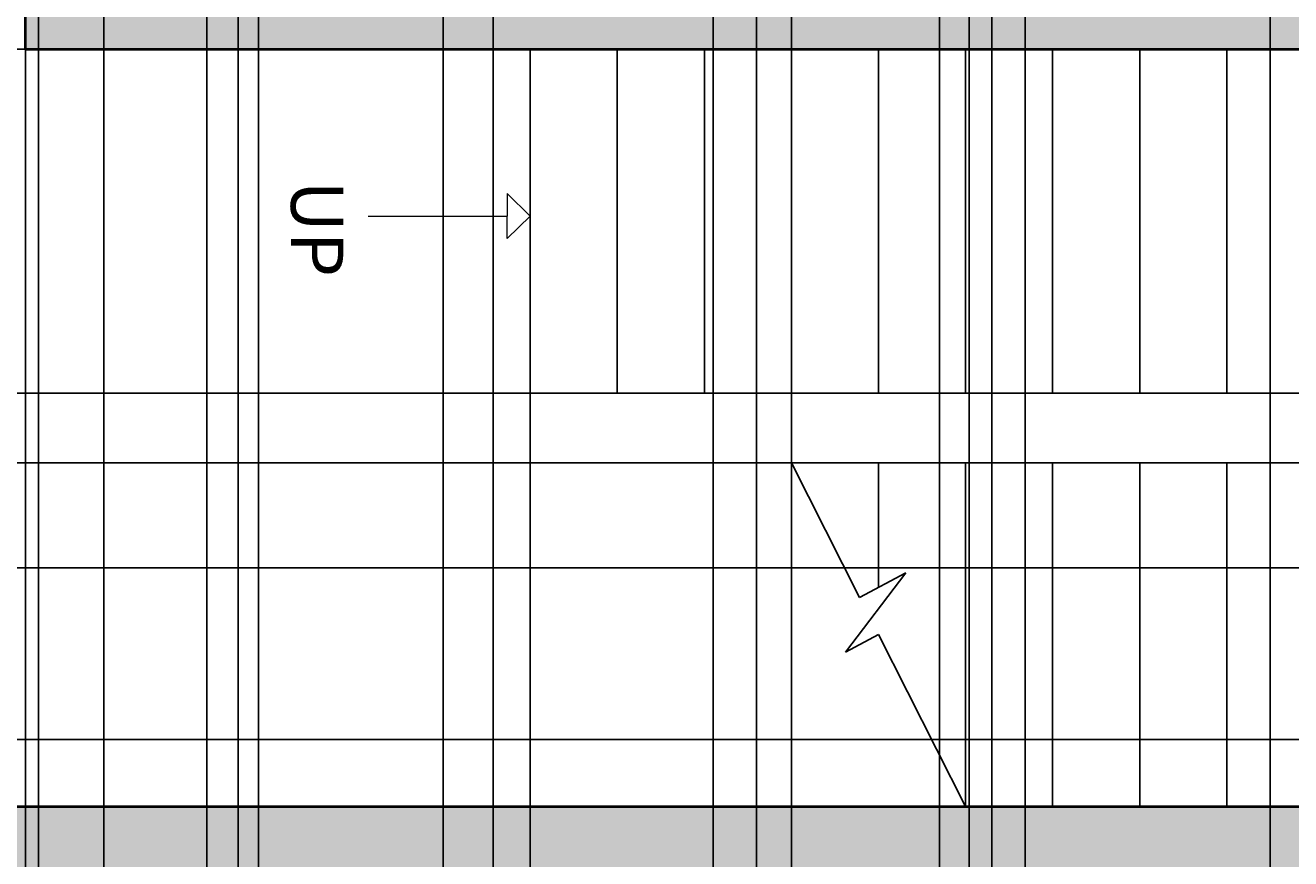
# Model space of a CAD drawing. Units: inches. Extents: x 818 to 1898, y 976 to 2364.
# Tile 48 of 96: x 1512 to 1657, y 1594 to 1690. Entities that reach past the tile are written whole.
import ezdxf

# ---------------------------------------------------------------- set-up
doc = ezdxf.new("R2010")
doc.units = ezdxf.units.IN
doc.header["$LTSCALE"] = 5
doc.header["$MEASUREMENT"] = 0
for name, color, linetype, lineweight in [('A-ANNO-DIMS', 2, 'Continuous', 18), ('A-ANNO-SYMB', 7, 'Continuous', 18), ('A-ANNO-TEXT', 7, 'Continuous', 18), ('A-FLOR-STRS', 7, 'Continuous', 25), ('A-WALL', 7, 'Continuous', 40)]:
    doc.layers.add(name, color=color, linetype=linetype, lineweight=lineweight)
doc.layers.add('A-WALL-PATT', color=251, linetype='Continuous', lineweight=13, true_color=0x636466)
doc.styles.get("Standard").update_dxf_attribs({"font": 'arial.ttf'})
doc.dimstyles.get("Standard").update_dxf_attribs({"dimtxt": 0.18, "dimasz": 0.18, "dimexe": 0.18, "dimexo": 0.0625, "dimgap": 0.09, "dimtad": 0, "dimtih": 1, "dimtoh": 1, "dimdec": 4, "dimzin": 0, "dimdsep": 46, "dimtxsty": 'Standard', "dimcen": 0.09, "dimadec": 0, "dimazin": 0, "dimtfac": 1, "dimtdec": 4, "dimtofl": 0, "dimtmove": 0, "dimatfit": 3, "dimfxl": 1, "dimtolj": 1, "dimtzin": 0, "dimarcsym": 0})

# ---------------------------------------------------------------- blocks, each defined once
blk = doc.blocks.new('*D101')
at = {"layer": 'A-ANNO-DIMS', "color": 0, "lineweight": -2, "ltscale": 5, "transparency": 16777216}
for p, q in [((1507.3, 1071.12), (1507.3, 2363.87)), ((1507.48, 2363.69), (1536, 2363.69)), ((1565.3, 2363.69), (1536.78, 2363.69)), ((1565.48, 1071.12), (1565.48, 2363.87))]:
    blk.add_line(p, q, dxfattribs=at)
at = {"layer": 'A-ANNO-DIMS', "color": 0, "ltscale": 5, "transparency": 16777216}
for points in [[(1507.48, 2363.72), (1507.48, 2363.66), (1507.3, 2363.69)], [(1565.3, 2363.72), (1565.3, 2363.66), (1565.48, 2363.69)]]:
    blk.add_solid(points, dxfattribs=at)
at = {"layer": 'Defpoints', "color": 0, "ltscale": 5, "transparency": 16777216}
for p in [(1565.48, 2363.69), (1507.3, 1071.06), (1565.48, 1071.06)]:
    blk.add_point(p, dxfattribs=at)
at = {"layer": 'A-ANNO-DIMS', "color": 0, "ltscale": 5, "transparency": 16777216, "insert": (1536.39, 2363.69), "char_height": 0.18, "attachment_point": 5}
blk.add_mtext('\\A1;58.19', dxfattribs=at)
blk = doc.blocks.new('*D102')
at = {"layer": 'A-ANNO-DIMS', "color": 0, "lineweight": -2, "ltscale": 5, "transparency": 16777216}
for p, q in [((1565.48, 1071.12), (1565.48, 2363.87)), ((1565.66, 2363.69), (1595.63, 2363.69)), ((1626.39, 2363.69), (1596.42, 2363.69)), ((1626.57, 1071.12), (1626.57, 2363.87))]:
    blk.add_line(p, q, dxfattribs=at)
at = {"layer": 'A-ANNO-DIMS', "color": 0, "ltscale": 5, "transparency": 16777216}
for points in [[(1565.66, 2363.72), (1565.66, 2363.66), (1565.48, 2363.69)], [(1626.39, 2363.72), (1626.39, 2363.66), (1626.57, 2363.69)]]:
    blk.add_solid(points, dxfattribs=at)
at = {"layer": 'Defpoints', "color": 0, "ltscale": 5, "transparency": 16777216}
for p in [(1626.57, 2363.69), (1565.48, 1071.06), (1626.57, 1071.06)]:
    blk.add_point(p, dxfattribs=at)
at = {"layer": 'A-ANNO-DIMS', "color": 0, "ltscale": 5, "transparency": 16777216, "insert": (1596.03, 2363.69), "char_height": 0.18, "attachment_point": 5}
blk.add_mtext('\\A1;61.09', dxfattribs=at)
blk = doc.blocks.new('*D103')
at = {"layer": 'A-ANNO-DIMS', "color": 0, "lineweight": -2, "ltscale": 5, "transparency": 16777216}
for p, q in [((1626.57, 1071.12), (1626.57, 2363.87)), ((1626.75, 2363.69), (1657.7, 2363.69)), ((1689.29, 2363.69), (1658.35, 2363.69)), ((1689.47, 1071.12), (1689.47, 2363.87))]:
    blk.add_line(p, q, dxfattribs=at)
at = {"layer": 'A-ANNO-DIMS', "color": 0, "ltscale": 5, "transparency": 16777216}
for points in [[(1626.75, 2363.72), (1626.75, 2363.66), (1626.57, 2363.69)], [(1689.29, 2363.72), (1689.29, 2363.66), (1689.47, 2363.69)]]:
    blk.add_solid(points, dxfattribs=at)
at = {"layer": 'Defpoints', "color": 0, "ltscale": 5, "transparency": 16777216}
for p in [(1689.47, 2363.69), (1626.57, 1071.06), (1689.47, 1071.06)]:
    blk.add_point(p, dxfattribs=at)
at = {"layer": 'A-ANNO-DIMS', "color": 0, "ltscale": 5, "transparency": 16777216, "insert": (1658.02, 2363.69), "char_height": 0.18, "attachment_point": 5}
blk.add_mtext('\\A1;62.9', dxfattribs=at)
blk = doc.blocks.new('*D118')
at = {"layer": 'A-ANNO-DIMS', "color": 0, "lineweight": -2, "ltscale": 5, "transparency": 16777216}
for p, q in [((1766.29, 1627.51), (818.03, 1627.51)), ((818.21, 1627.33), (818.21, 1586.53)), ((818.21, 1545.36), (818.21, 1586.16)), ((1766.29, 1545.18), (818.03, 1545.18))]:
    blk.add_line(p, q, dxfattribs=at)
at = {"layer": 'A-ANNO-DIMS', "color": 0, "ltscale": 5, "transparency": 16777216}
for points in [[(818.18, 1627.33), (818.24, 1627.33), (818.21, 1627.51)], [(818.18, 1545.36), (818.24, 1545.36), (818.21, 1545.18)]]:
    blk.add_solid(points, dxfattribs=at)
at = {"layer": 'Defpoints', "color": 0, "ltscale": 5, "transparency": 16777216}
for p in [(818.21, 1627.51), (1766.35, 1627.51), (1766.35, 1545.18)]:
    blk.add_point(p, dxfattribs=at)
at = {"layer": 'A-ANNO-DIMS', "color": 0, "ltscale": 5, "transparency": 16777216, "insert": (818.21, 1586.34), "char_height": 0.18, "attachment_point": 5}
blk.add_mtext('\\A1;82.32', dxfattribs=at)
blk = doc.blocks.new('*D119')
at = {"layer": 'A-ANNO-DIMS', "color": 0, "lineweight": -2, "ltscale": 5, "transparency": 16777216}
for p, q in [((1766.29, 1716.99), (818.03, 1716.99)), ((818.21, 1716.81), (818.21, 1672.43)), ((818.21, 1627.69), (818.21, 1672.06)), ((1766.29, 1627.51), (818.03, 1627.51))]:
    blk.add_line(p, q, dxfattribs=at)
at = {"layer": 'A-ANNO-DIMS', "color": 0, "ltscale": 5, "transparency": 16777216}
for points in [[(818.18, 1716.81), (818.24, 1716.81), (818.21, 1716.99)], [(818.18, 1627.69), (818.24, 1627.69), (818.21, 1627.51)]]:
    blk.add_solid(points, dxfattribs=at)
at = {"layer": 'Defpoints', "color": 0, "ltscale": 5, "transparency": 16777216}
for p in [(818.21, 1716.99), (1766.35, 1716.99), (1766.35, 1627.51)]:
    blk.add_point(p, dxfattribs=at)
at = {"layer": 'A-ANNO-DIMS', "color": 0, "ltscale": 5, "transparency": 16777216, "insert": (818.21, 1672.25), "char_height": 0.18, "attachment_point": 5}
blk.add_mtext('\\A1;89.48', dxfattribs=at)
blk = doc.blocks.new('*D170')
at = {"layer": 'A-ANNO-DIMS', "color": 0, "lineweight": -2, "ltscale": 5, "transparency": 16777216}
for p, q in [((1430.79, 1600.08), (1897.92, 1600.08)), ((1897.74, 1599.9), (1897.74, 1550.76)), ((1897.74, 1501.26), (1897.74, 1550.4)), ((1430.79, 1501.08), (1897.92, 1501.08))]:
    blk.add_line(p, q, dxfattribs=at)
at = {"layer": 'A-ANNO-DIMS', "color": 0, "ltscale": 5, "transparency": 16777216}
for points in [[(1897.71, 1599.9), (1897.77, 1599.9), (1897.74, 1600.08)], [(1897.71, 1501.26), (1897.77, 1501.26), (1897.74, 1501.08)]]:
    blk.add_solid(points, dxfattribs=at)
at = {"layer": 'Defpoints', "color": 0, "ltscale": 5, "transparency": 16777216}
for p in [(1430.73, 1600.08), (1897.74, 1600.08), (1430.73, 1501.08)]:
    blk.add_point(p, dxfattribs=at)
at = {"layer": 'A-ANNO-DIMS', "color": 0, "ltscale": 5, "transparency": 16777216, "insert": (1897.74, 1550.58), "char_height": 0.18, "attachment_point": 5}
blk.add_mtext('\\A1;99', dxfattribs=at)
blk = doc.blocks.new('*D173')
at = {"layer": 'A-ANNO-DIMS', "color": 0, "lineweight": -2, "ltscale": 5, "transparency": 16777216}
for p, q in [((1622.73, 1463.14), (1622.73, 2363.87)), ((1622.91, 2363.69), (1638.51, 2363.69)), ((1654.55, 2363.69), (1638.94, 2363.69)), ((1654.73, 1463.14), (1654.73, 2363.87))]:
    blk.add_line(p, q, dxfattribs=at)
at = {"layer": 'A-ANNO-DIMS', "color": 0, "ltscale": 5, "transparency": 16777216}
for points in [[(1622.91, 2363.72), (1622.91, 2363.66), (1622.73, 2363.69)], [(1654.55, 2363.72), (1654.55, 2363.66), (1654.73, 2363.69)]]:
    blk.add_solid(points, dxfattribs=at)
at = {"layer": 'Defpoints', "color": 0, "ltscale": 5, "transparency": 16777216}
for p in [(1654.73, 2363.69), (1622.73, 1463.08), (1654.73, 1463.08)]:
    blk.add_point(p, dxfattribs=at)
at = {"layer": 'A-ANNO-DIMS', "color": 0, "ltscale": 5, "transparency": 16777216, "insert": (1638.73, 2363.69), "char_height": 0.18, "attachment_point": 5}
blk.add_mtext('\\A1;32', dxfattribs=at)
blk = doc.blocks.new('*D174')
at = {"layer": 'A-ANNO-DIMS', "color": 0, "lineweight": -2, "ltscale": 5, "transparency": 16777216}
for p, q in [((1616.73, 1416.75), (1616.73, 2363.87)), ((1616.91, 2363.69), (1619.58, 2363.69)), ((1622.55, 2363.69), (1619.87, 2363.69)), ((1622.73, 1416.75), (1622.73, 2363.87))]:
    blk.add_line(p, q, dxfattribs=at)
at = {"layer": 'A-ANNO-DIMS', "color": 0, "ltscale": 5, "transparency": 16777216}
for points in [[(1616.91, 2363.72), (1616.91, 2363.66), (1616.73, 2363.69)], [(1622.55, 2363.72), (1622.55, 2363.66), (1622.73, 2363.69)]]:
    blk.add_solid(points, dxfattribs=at)
at = {"layer": 'Defpoints', "color": 0, "ltscale": 5, "transparency": 16777216}
for p in [(1622.73, 2363.69), (1616.73, 1416.69), (1622.73, 1416.69)]:
    blk.add_point(p, dxfattribs=at)
at = {"layer": 'A-ANNO-DIMS', "color": 0, "ltscale": 5, "transparency": 16777216, "insert": (1619.73, 2363.69), "char_height": 0.18, "attachment_point": 5}
blk.add_mtext('\\A1;6', dxfattribs=at)
blk = doc.blocks.new('*D175')
at = {"layer": 'A-ANNO-DIMS', "color": 0, "lineweight": -2, "ltscale": 5, "transparency": 16777216}
for p, q in [((1559.73, 1647.64), (1559.73, 2363.87)), ((1559.91, 2363.69), (1614.45, 2363.69)), ((1669.55, 2363.69), (1615.01, 2363.69)), ((1669.73, 1647.64), (1669.73, 2363.87))]:
    blk.add_line(p, q, dxfattribs=at)
at = {"layer": 'A-ANNO-DIMS', "color": 0, "ltscale": 5, "transparency": 16777216}
for points in [[(1559.91, 2363.72), (1559.91, 2363.66), (1559.73, 2363.69)], [(1669.55, 2363.72), (1669.55, 2363.66), (1669.73, 2363.69)]]:
    blk.add_solid(points, dxfattribs=at)
at = {"layer": 'Defpoints', "color": 0, "ltscale": 5, "transparency": 16777216}
for p in [(1669.73, 2363.69), (1559.73, 1647.58), (1669.73, 1647.58)]:
    blk.add_point(p, dxfattribs=at)
at = {"layer": 'A-ANNO-DIMS', "color": 0, "ltscale": 5, "transparency": 16777216, "insert": (1614.73, 2363.69), "char_height": 0.18, "attachment_point": 5}
blk.add_mtext('\\A1;110', dxfattribs=at)
blk = doc.blocks.new('*D176')
at = {"layer": 'A-ANNO-DIMS', "color": 0, "lineweight": -2, "ltscale": 5, "transparency": 16777216}
for p, q in [((1559.66, 1687.08), (818.03, 1687.08)), ((818.21, 1686.9), (818.21, 1667.51)), ((818.21, 1647.76), (818.21, 1667.15)), ((1559.66, 1647.58), (818.03, 1647.58))]:
    blk.add_line(p, q, dxfattribs=at)
at = {"layer": 'A-ANNO-DIMS', "color": 0, "ltscale": 5, "transparency": 16777216}
for points in [[(818.18, 1686.9), (818.24, 1686.9), (818.21, 1687.08)], [(818.18, 1647.76), (818.24, 1647.76), (818.21, 1647.58)]]:
    blk.add_solid(points, dxfattribs=at)
at = {"layer": 'Defpoints', "color": 0, "ltscale": 5, "transparency": 16777216}
for p in [(1559.73, 1687.08), (818.21, 1647.58), (1559.73, 1647.58)]:
    blk.add_point(p, dxfattribs=at)
at = {"layer": 'A-ANNO-DIMS', "color": 0, "ltscale": 5, "transparency": 16777216, "insert": (818.21, 1667.33), "char_height": 0.18, "attachment_point": 5}
blk.add_mtext('\\A1;39.5', dxfattribs=at)
blk = doc.blocks.new('*D177')
at = {"layer": 'A-ANNO-DIMS', "color": 0, "lineweight": -2, "ltscale": 5, "transparency": 16777216}
for p, q in [((1559.73, 1647.52), (1559.73, 975.66)), ((1569.73, 1647.52), (1569.73, 975.66)), ((1559.91, 975.84), (1564.52, 975.84)), ((1569.55, 975.84), (1564.94, 975.84))]:
    blk.add_line(p, q, dxfattribs=at)
at = {"layer": 'A-ANNO-DIMS', "color": 0, "ltscale": 5, "transparency": 16777216}
for points in [[(1559.91, 975.87), (1559.91, 975.81), (1559.73, 975.84)], [(1569.55, 975.87), (1569.55, 975.81), (1569.73, 975.84)]]:
    blk.add_solid(points, dxfattribs=at)
at = {"layer": 'Defpoints', "color": 0, "ltscale": 5, "transparency": 16777216}
for p in [(1559.73, 1647.58), (1569.73, 1647.58), (1569.73, 975.84)]:
    blk.add_point(p, dxfattribs=at)
at = {"layer": 'A-ANNO-DIMS', "color": 0, "ltscale": 5, "transparency": 16777216, "insert": (1564.73, 975.84), "char_height": 0.18, "attachment_point": 5}
blk.add_mtext('\\A1;10', dxfattribs=at)
blk = doc.blocks.new('*D180')
at = {"layer": 'A-ANNO-DIMS', "color": 0, "lineweight": -2, "ltscale": 5, "transparency": 16777216}
for p, q in [((1599.73, 1639.52), (1599.73, 975.66)), ((1669.73, 1639.52), (1669.73, 975.66)), ((1599.91, 975.84), (1634.51, 975.84)), ((1669.55, 975.84), (1634.94, 975.84))]:
    blk.add_line(p, q, dxfattribs=at)
at = {"layer": 'A-ANNO-DIMS', "color": 0, "ltscale": 5, "transparency": 16777216}
for points in [[(1599.91, 975.87), (1599.91, 975.81), (1599.73, 975.84)], [(1669.55, 975.87), (1669.55, 975.81), (1669.73, 975.84)]]:
    blk.add_solid(points, dxfattribs=at)
at = {"layer": 'Defpoints', "color": 0, "ltscale": 5, "transparency": 16777216}
for p in [(1599.73, 1639.58), (1669.73, 1639.58), (1669.73, 975.84)]:
    blk.add_point(p, dxfattribs=at)
at = {"layer": 'A-ANNO-DIMS', "color": 0, "ltscale": 5, "transparency": 16777216, "insert": (1634.73, 975.84), "char_height": 0.18, "attachment_point": 5}
blk.add_mtext('\\A1;70', dxfattribs=at)
blk = doc.blocks.new('*D181')
at = {"layer": 'A-ANNO-DIMS', "color": 0, "lineweight": -2, "ltscale": 5, "transparency": 16777216}
for p, q in [((1599.66, 1639.58), (818.03, 1639.58)), ((818.21, 1639.4), (818.21, 1620.01)), ((818.21, 1600.26), (818.21, 1619.65)), ((1619.66, 1600.08), (818.03, 1600.08))]:
    blk.add_line(p, q, dxfattribs=at)
at = {"layer": 'A-ANNO-DIMS', "color": 0, "ltscale": 5, "transparency": 16777216}
for points in [[(818.18, 1639.4), (818.24, 1639.4), (818.21, 1639.58)], [(818.18, 1600.26), (818.24, 1600.26), (818.21, 1600.08)]]:
    blk.add_solid(points, dxfattribs=at)
at = {"layer": 'Defpoints', "color": 0, "ltscale": 5, "transparency": 16777216}
for p in [(1599.73, 1639.58), (818.21, 1600.08), (1619.73, 1600.08)]:
    blk.add_point(p, dxfattribs=at)
at = {"layer": 'A-ANNO-DIMS', "color": 0, "ltscale": 5, "transparency": 16777216, "insert": (818.21, 1619.83), "char_height": 0.18, "attachment_point": 5}
blk.add_mtext('\\A1;39.5', dxfattribs=at)
blk = doc.blocks.new('*D182')
at = {"layer": 'A-ANNO-DIMS', "color": 0, "lineweight": -2, "ltscale": 5, "transparency": 16777216}
for p, q in [((1463.73, 1687.02), (1463.73, 975.66)), ((1559.73, 1687.02), (1559.73, 975.66)), ((1463.91, 975.84), (1511.51, 975.84)), ((1559.55, 975.84), (1511.94, 975.84))]:
    blk.add_line(p, q, dxfattribs=at)
at = {"layer": 'A-ANNO-DIMS', "color": 0, "ltscale": 5, "transparency": 16777216}
for points in [[(1463.91, 975.87), (1463.91, 975.81), (1463.73, 975.84)], [(1559.55, 975.87), (1559.55, 975.81), (1559.73, 975.84)]]:
    blk.add_solid(points, dxfattribs=at)
at = {"layer": 'Defpoints', "color": 0, "ltscale": 5, "transparency": 16777216}
for p in [(1463.73, 1687.08), (1559.73, 1687.08), (1559.73, 975.84)]:
    blk.add_point(p, dxfattribs=at)
at = {"layer": 'A-ANNO-DIMS', "color": 0, "ltscale": 5, "transparency": 16777216, "insert": (1511.73, 975.84), "char_height": 0.18, "attachment_point": 5}
blk.add_mtext('\\A1;96', dxfattribs=at)
blk = doc.blocks.new('*D199')
at = {"layer": 'A-ANNO-DIMS', "color": 0, "lineweight": -2, "ltscale": 5, "transparency": 16777216}
for p, q in [((1559.79, 1687.08), (1897.92, 1687.08)), ((1897.74, 1686.9), (1897.74, 1513.15)), ((1897.74, 1339.05), (1897.74, 1512.79)), ((1660.38, 1338.87), (1897.92, 1338.87))]:
    blk.add_line(p, q, dxfattribs=at)
at = {"layer": 'A-ANNO-DIMS', "color": 0, "ltscale": 5, "transparency": 16777216}
for points in [[(1897.71, 1686.9), (1897.77, 1686.9), (1897.74, 1687.08)], [(1897.71, 1339.05), (1897.77, 1339.05), (1897.74, 1338.87)]]:
    blk.add_solid(points, dxfattribs=at)
at = {"layer": 'Defpoints', "color": 0, "ltscale": 5, "transparency": 16777216}
for p in [(1559.73, 1687.08), (1897.74, 1687.08), (1660.31, 1338.87)]:
    blk.add_point(p, dxfattribs=at)
at = {"layer": 'A-ANNO-DIMS', "color": 0, "ltscale": 5, "transparency": 16777216, "insert": (1897.74, 1512.97), "char_height": 0.18, "attachment_point": 5}
blk.add_mtext('\\A1;348.2', dxfattribs=at)
blk = doc.blocks.new('*D214')
at = {"layer": 'A-ANNO-DIMS', "color": 0, "lineweight": -2, "ltscale": 5, "transparency": 16777216}
for p, q in [((1511.73, 1687.02), (1511.73, 975.66)), ((1714.73, 1687.02), (1714.73, 975.66)), ((1511.91, 975.84), (1612.93, 975.84)), ((1714.55, 975.84), (1613.52, 975.84))]:
    blk.add_line(p, q, dxfattribs=at)
at = {"layer": 'A-ANNO-DIMS', "color": 0, "ltscale": 5, "transparency": 16777216}
for points in [[(1511.91, 975.87), (1511.91, 975.81), (1511.73, 975.84)], [(1714.55, 975.87), (1714.55, 975.81), (1714.73, 975.84)]]:
    blk.add_solid(points, dxfattribs=at)
at = {"layer": 'Defpoints', "color": 0, "ltscale": 5, "transparency": 16777216}
for p in [(1511.73, 1687.08), (1714.73, 1687.08), (1714.73, 975.84)]:
    blk.add_point(p, dxfattribs=at)
at = {"layer": 'A-ANNO-DIMS', "color": 0, "ltscale": 5, "transparency": 16777216, "insert": (1613.23, 975.84), "char_height": 0.18, "attachment_point": 5}
blk.add_mtext('\\A1;203', dxfattribs=at)
blk = doc.blocks.new('*D215')
at = {"layer": 'A-ANNO-DIMS', "color": 0, "lineweight": -2, "ltscale": 5, "transparency": 16777216}
for p, q in [((1590.66, 1876.08), (818.03, 1876.08)), ((818.21, 1875.9), (818.21, 1781.76)), ((818.21, 1687.26), (818.21, 1781.4)), ((1511.66, 1687.08), (818.03, 1687.08))]:
    blk.add_line(p, q, dxfattribs=at)
at = {"layer": 'A-ANNO-DIMS', "color": 0, "ltscale": 5, "transparency": 16777216}
for points in [[(818.18, 1875.9), (818.24, 1875.9), (818.21, 1876.08)], [(818.18, 1687.26), (818.24, 1687.26), (818.21, 1687.08)]]:
    blk.add_solid(points, dxfattribs=at)
at = {"layer": 'Defpoints', "color": 0, "ltscale": 5, "transparency": 16777216}
for p in [(818.21, 1876.08), (1590.73, 1876.08), (1511.73, 1687.08)]:
    blk.add_point(p, dxfattribs=at)
at = {"layer": 'A-ANNO-DIMS', "color": 0, "ltscale": 5, "transparency": 16777216, "insert": (818.21, 1781.58), "char_height": 0.18, "attachment_point": 5}
blk.add_mtext('\\A1;189', dxfattribs=at)
blk = doc.blocks.new('*D219')
at = {"layer": 'A-ANNO-DIMS', "color": 0, "lineweight": -2, "ltscale": 5, "transparency": 16777216}
for p, q in [((1595.73, 1696.02), (1595.73, 975.66)), ((1599.73, 1696.02), (1599.73, 975.66)), ((1595.91, 975.84), (1597.57, 975.84)), ((1599.55, 975.84), (1597.88, 975.84))]:
    blk.add_line(p, q, dxfattribs=at)
at = {"layer": 'A-ANNO-DIMS', "color": 0, "ltscale": 5, "transparency": 16777216}
for points in [[(1595.91, 975.87), (1595.91, 975.81), (1595.73, 975.84)], [(1599.55, 975.87), (1599.55, 975.81), (1599.73, 975.84)]]:
    blk.add_solid(points, dxfattribs=at)
at = {"layer": 'Defpoints', "color": 0, "ltscale": 5, "transparency": 16777216}
for p in [(1595.73, 1696.08), (1599.73, 1696.08), (1599.73, 975.84)]:
    blk.add_point(p, dxfattribs=at)
at = {"layer": 'A-ANNO-DIMS', "color": 0, "ltscale": 5, "transparency": 16777216, "insert": (1597.73, 975.84), "char_height": 0.18, "attachment_point": 5}
blk.add_mtext('\\A1;4', dxfattribs=at)
blk = doc.blocks.new('*D224')
at = {"layer": 'A-ANNO-DIMS', "color": 0, "lineweight": -2, "ltscale": 5, "transparency": 16777216}
for p, q in [((1520.73, 1837.52), (1520.73, 975.66)), ((1532.59, 1837.52), (1532.59, 975.66)), ((1520.91, 975.84), (1526.2, 975.84)), ((1532.41, 975.84), (1527.11, 975.84))]:
    blk.add_line(p, q, dxfattribs=at)
at = {"layer": 'A-ANNO-DIMS', "color": 0, "ltscale": 5, "transparency": 16777216}
for points in [[(1520.91, 975.87), (1520.91, 975.81), (1520.73, 975.84)], [(1532.41, 975.87), (1532.41, 975.81), (1532.59, 975.84)]]:
    blk.add_solid(points, dxfattribs=at)
at = {"layer": 'Defpoints', "color": 0, "ltscale": 5, "transparency": 16777216}
for p in [(1520.73, 1837.58), (1532.59, 1837.58), (1532.59, 975.84)]:
    blk.add_point(p, dxfattribs=at)
at = {"layer": 'A-ANNO-DIMS', "color": 0, "ltscale": 5, "transparency": 16777216, "insert": (1526.66, 975.84), "char_height": 0.18, "attachment_point": 5}
blk.add_mtext('\\A1;11.868', dxfattribs=at)
blk = doc.blocks.new('*D226')
at = {"layer": 'A-ANNO-DIMS', "color": 0, "lineweight": -2, "ltscale": 5, "transparency": 16777216}
for p, q in [((1536.17, 1774.47), (1536.17, 975.66)), ((1520.73, 1773.02), (1520.73, 975.66)), ((1520.91, 975.84), (1527.99, 975.84)), ((1535.99, 975.84), (1528.9, 975.84))]:
    blk.add_line(p, q, dxfattribs=at)
at = {"layer": 'A-ANNO-DIMS', "color": 0, "ltscale": 5, "transparency": 16777216}
for points in [[(1520.91, 975.87), (1520.91, 975.81), (1520.73, 975.84)], [(1535.99, 975.87), (1535.99, 975.81), (1536.17, 975.84)]]:
    blk.add_solid(points, dxfattribs=at)
at = {"layer": 'Defpoints', "color": 0, "ltscale": 5, "transparency": 16777216}
for p in [(1536.17, 1774.53), (1520.73, 1773.08), (1536.17, 975.84)]:
    blk.add_point(p, dxfattribs=at)
at = {"layer": 'A-ANNO-DIMS', "color": 0, "ltscale": 5, "transparency": 16777216, "insert": (1528.45, 975.84), "char_height": 0.18, "attachment_point": 5}
blk.add_mtext('\\A1;15.445', dxfattribs=at)
blk = doc.blocks.new('*D229')
at = {"layer": 'A-ANNO-DIMS', "color": 0, "lineweight": -2, "ltscale": 5, "transparency": 16777216}
for p, q in [((1599.73, 2044.02), (1599.73, 975.66)), ((1620.14, 2036.06), (1620.14, 975.66)), ((1599.91, 975.84), (1609.47, 975.84)), ((1619.96, 975.84), (1610.4, 975.84))]:
    blk.add_line(p, q, dxfattribs=at)
at = {"layer": 'A-ANNO-DIMS', "color": 0, "ltscale": 5, "transparency": 16777216}
for points in [[(1599.91, 975.87), (1599.91, 975.81), (1599.73, 975.84)], [(1619.96, 975.87), (1619.96, 975.81), (1620.14, 975.84)]]:
    blk.add_solid(points, dxfattribs=at)
at = {"layer": 'Defpoints', "color": 0, "ltscale": 5, "transparency": 16777216}
for p in [(1599.73, 2044.08), (1620.14, 2036.12), (1620.14, 975.84)]:
    blk.add_point(p, dxfattribs=at)
at = {"layer": 'A-ANNO-DIMS', "color": 0, "ltscale": 5, "transparency": 16777216, "insert": (1609.93, 975.84), "char_height": 0.18, "attachment_point": 5}
blk.add_mtext('\\A1;20.416', dxfattribs=at)
blk = doc.blocks.new('*D242')
at = {"layer": 'A-ANNO-DIMS', "color": 0, "lineweight": -2, "ltscale": 5, "transparency": 16777216}
for p, q in [((1488.26, 1948.6), (1488.26, 975.66)), ((1513.23, 1948.6), (1513.23, 975.66)), ((1488.44, 975.84), (1500.35, 975.84)), ((1513.05, 975.84), (1501.14, 975.84))]:
    blk.add_line(p, q, dxfattribs=at)
at = {"layer": 'A-ANNO-DIMS', "color": 0, "ltscale": 5, "transparency": 16777216}
for points in [[(1488.44, 975.87), (1488.44, 975.81), (1488.26, 975.84)], [(1513.05, 975.87), (1513.05, 975.81), (1513.23, 975.84)]]:
    blk.add_solid(points, dxfattribs=at)
at = {"layer": 'Defpoints', "color": 0, "ltscale": 5, "transparency": 16777216}
for p in [(1488.26, 1948.66), (1513.23, 1948.66), (1513.23, 975.84)]:
    blk.add_point(p, dxfattribs=at)
at = {"layer": 'A-ANNO-DIMS', "color": 0, "ltscale": 5, "transparency": 16777216, "insert": (1500.74, 975.84), "char_height": 0.18, "attachment_point": 5}
blk.add_mtext('\\A1;24.97', dxfattribs=at)
blk = doc.blocks.new('*D243')
at = {"layer": 'A-ANNO-DIMS', "color": 0, "lineweight": -2, "ltscale": 5, "transparency": 16777216}
for p, q in [((1451.77, 2020.02), (1451.77, 975.66)), ((1590.73, 2020.02), (1590.73, 975.66)), ((1451.95, 975.84), (1520.79, 975.84)), ((1590.55, 975.84), (1521.7, 975.84))]:
    blk.add_line(p, q, dxfattribs=at)
at = {"layer": 'A-ANNO-DIMS', "color": 0, "ltscale": 5, "transparency": 16777216}
for points in [[(1451.95, 975.87), (1451.95, 975.81), (1451.77, 975.84)], [(1590.55, 975.87), (1590.55, 975.81), (1590.73, 975.84)]]:
    blk.add_solid(points, dxfattribs=at)
at = {"layer": 'Defpoints', "color": 0, "ltscale": 5, "transparency": 16777216}
for p in [(1451.77, 2020.08), (1590.73, 2020.08), (1590.73, 975.84)]:
    blk.add_point(p, dxfattribs=at)
at = {"layer": 'A-ANNO-DIMS', "color": 0, "ltscale": 5, "transparency": 16777216, "insert": (1521.25, 975.84), "char_height": 0.18, "attachment_point": 5}
blk.add_mtext('\\A1;138.96', dxfattribs=at)
blk = doc.blocks.new('*D253')
at = {"layer": 'A-ANNO-DIMS', "color": 0, "lineweight": -2, "ltscale": 5, "transparency": 16777216}
for p, q in [((1485.12, 2053.02), (1485.12, 975.66)), ((1538.52, 2053.02), (1538.52, 975.66)), ((1485.3, 975.84), (1511.42, 975.84)), ((1538.34, 975.84), (1512.21, 975.84))]:
    blk.add_line(p, q, dxfattribs=at)
at = {"layer": 'A-ANNO-DIMS', "color": 0, "ltscale": 5, "transparency": 16777216}
for points in [[(1485.3, 975.87), (1485.3, 975.81), (1485.12, 975.84)], [(1538.34, 975.87), (1538.34, 975.81), (1538.52, 975.84)]]:
    blk.add_solid(points, dxfattribs=at)
at = {"layer": 'Defpoints', "color": 0, "ltscale": 5, "transparency": 16777216}
for p in [(1485.12, 2053.08), (1538.52, 2053.08), (1538.52, 975.84)]:
    blk.add_point(p, dxfattribs=at)
at = {"layer": 'A-ANNO-DIMS', "color": 0, "ltscale": 5, "transparency": 16777216, "insert": (1511.82, 975.84), "char_height": 0.18, "attachment_point": 5}
blk.add_mtext('\\A1;53.39', dxfattribs=at)
blk = doc.blocks.new('*D282')
at = {"layer": 'A-ANNO-DIMS', "color": 0, "lineweight": -2, "ltscale": 5, "transparency": 16777216}
for p, q in [((1422.08, 2081.19), (1897.92, 2081.19)), ((1897.74, 2081.01), (1897.74, 1884.32)), ((1897.74, 1687.26), (1897.74, 1883.95)), ((1463.79, 1687.08), (1897.92, 1687.08))]:
    blk.add_line(p, q, dxfattribs=at)
at = {"layer": 'A-ANNO-DIMS', "color": 0, "ltscale": 5, "transparency": 16777216}
for points in [[(1897.71, 2081.01), (1897.77, 2081.01), (1897.74, 2081.19)], [(1897.71, 1687.26), (1897.77, 1687.26), (1897.74, 1687.08)]]:
    blk.add_solid(points, dxfattribs=at)
at = {"layer": 'Defpoints', "color": 0, "ltscale": 5, "transparency": 16777216}
for p in [(1422.02, 2081.19), (1897.74, 2081.19), (1463.73, 1687.08)]:
    blk.add_point(p, dxfattribs=at)
at = {"layer": 'A-ANNO-DIMS', "color": 0, "ltscale": 5, "transparency": 16777216, "insert": (1897.74, 1884.13), "char_height": 0.18, "attachment_point": 5}
blk.add_mtext('\\A1;394.1', dxfattribs=at)
blk = doc.blocks.new('*D291')
at = {"layer": 'A-ANNO-DIMS', "color": 0, "lineweight": -2, "ltscale": 5, "transparency": 16777216}
for p, q in [((1206.79, 1687.08), (1897.92, 1687.08)), ((1897.74, 1686.9), (1897.74, 1647.61)), ((1897.74, 1607.95), (1897.74, 1647.24)), ((1318.96, 1607.77), (1897.92, 1607.77))]:
    blk.add_line(p, q, dxfattribs=at)
at = {"layer": 'A-ANNO-DIMS', "color": 0, "ltscale": 5, "transparency": 16777216}
for points in [[(1897.71, 1686.9), (1897.77, 1686.9), (1897.74, 1687.08)], [(1897.71, 1607.95), (1897.77, 1607.95), (1897.74, 1607.77)]]:
    blk.add_solid(points, dxfattribs=at)
at = {"layer": 'Defpoints', "color": 0, "ltscale": 5, "transparency": 16777216}
for p in [(1206.73, 1687.08), (1897.74, 1687.08), (1318.89, 1607.77)]:
    blk.add_point(p, dxfattribs=at)
at = {"layer": 'A-ANNO-DIMS', "color": 0, "ltscale": 5, "transparency": 16777216, "insert": (1897.74, 1647.42), "char_height": 0.18, "attachment_point": 5}
blk.add_mtext('\\A1;79.3', dxfattribs=at)

msp = doc.modelspace()

# ---------------------------------------------------------------- hatches: boundary and pattern name
at = {"layer": 'A-WALL-PATT', "ltscale": 5}
h = msp.add_hatch(color=256, dxfattribs=at)
h.dxf.hatch_style = 1
h.paths.add_polyline_path([(1267.7252, 1928.9218), (1258.7252, 1928.9218), (1258.7252, 1913.6401), (1250.3029, 1913.6401), (1250.3029, 1878.3919), (1258.7252, 1878.3919), (1258.7252, 1862.9652), (1267.7252, 1862.9652)])
h.paths.add_polyline_path([(1267.7252, 1814.9652), (1258.7252, 1814.9652), (1258.7252, 1755.3321), (1267.7252, 1755.3321)])
h.paths.add_polyline_path([(1463.7251, 1696.0782), (1267.7252, 1696.0782), (1267.7252, 1707.3321), (1258.7252, 1707.3321), (1258.7252, 1700.0782), (1251.9333, 1700.0782), (1251.9333, 1687.0782), (1463.7251, 1687.0782)])
h.paths.add_polyline_path([(1714.7251, 1717.3178), (1705.7252, 1717.3178), (1705.7252, 1696.0782), (1599.7251, 1696.0782), (1599.7251, 1790.0782), (1705.7252, 1790.0782), (1705.7252, 1785.6125), (1714.7251, 1785.6125), (1714.7251, 1827.2125), (1705.7252, 1827.2125), (1705.7252, 1802.0782), (1599.7251, 1802.0782), (1599.7251, 1867.0782), (1705.7252, 1867.0782), (1705.7252, 1857.2125), (1714.7251, 1857.2125), (1714.7251, 1930.0316), (1741.8409, 1930.0316), (1741.8409, 1935.0316), (1714.7251, 1935.0316), (1714.7251, 1957.0338), (1741.8409, 1957.0338), (1741.8409, 1962.0338), (1714.7251, 1962.0338), (1705.7252, 1962.0338), (1705.7252, 1948.0782), (1599.7251, 1948.0782), (1599.7251, 1981.0782), (1590.7251, 1981.0782), (1590.7251, 1941.0782), (1620.7252, 1941.0782), (1705.7252, 1941.0782), (1705.7252, 1876.0782), (1599.7251, 1876.0782), (1599.7251, 1911.0782), (1590.7251, 1911.0782), (1590.7251, 1876.0782), (1429.2252, 1876.0782), (1429.2252, 1867.0782), (1511.7251, 1867.0782), (1528.593, 1867.0782), (1595.7251, 1867.0782), (1595.7251, 1773.0782), (1520.7251, 1773.0782), (1520.7251, 1837.5823), (1532.593, 1837.5823), (1532.593, 1867.0782), (1528.593, 1867.0782), (1528.593, 1841.5823), (1511.7251, 1841.5823), (1511.7251, 1744.9714), (1520.7251, 1744.9714), (1520.7251, 1761.0782), (1595.7251, 1761.0782), (1595.7251, 1696.0782), (1520.7251, 1696.0782), (1520.7251, 1716.0454), (1511.7251, 1716.0454), (1511.7251, 1696.0782), (1511.7251, 1687.0782), (1714.7251, 1687.0782)])
h.paths.add_polyline_path([(1714.7251, 2053.0782), (1714.7251, 2081.1881), (1709.7252, 2081.1881), (1709.7252, 2053.0782), (1681.6446, 2053.0782), (1681.6446, 2081.1881), (1676.6446, 2081.1881), (1676.6446, 2053.0782), (1538.5155, 2053.0782), (1538.5155, 2044.0782), (1590.7251, 2044.0782), (1590.7251, 2011.0782), (1599.7251, 2011.0782), (1599.7251, 2044.0782), (1705.7252, 2044.0782), (1705.7252, 2014.5114), (1714.7251, 2014.5114)])
h.paths.add_polyline_path([(1485.1216, 2053.0782), (1422.02, 2053.0782), (1422.02, 2081.1881), (1413.02, 2081.1881), (1413.02, 2053.0782), (1399.6356, 2053.0782), (1399.6356, 2081.1881), (1390.6356, 2081.1881), (1390.6356, 2053.0782), (1388.0315, 2053.0782), (1388.0315, 2044.0782), (1416.2743, 2044.0782), (1485.1216, 2044.0782)])
h.paths.add_polyline_path([(1330.305, 2053.0782), (1258.7252, 2053.0782), (1258.7252, 2019.2871), (1267.7252, 2019.2871), (1267.7252, 2044.0782), (1330.305, 2044.0782)])
h.paths.add_polyline_path([(1258.7252, 2053.0782), (1214.6577, 2053.0782), (1214.6577, 2044.0782), (1258.7252, 2044.0782)])
h.paths.add_polyline_path([(1214.6577, 2053.0782), (1180.349, 2053.0782), (1180.349, 2044.0782), (1214.6577, 2044.0782)])
h.paths.add_polyline_path([(1714.7251, 1639.5782), (1741.8409, 1639.5782), (1741.8409, 1643.5782), (1714.7251, 1643.5782), (1714.7251, 1649.9029), (1705.7252, 1649.9029), (1705.7252, 1600.0782), (1477.7252, 1600.0782), (1477.7252, 1591.0782), (1520.7251, 1591.0782), (1616.7251, 1591.0782), (1616.7251, 1416.6857), (1622.7251, 1416.6857), (1622.7251, 1463.0782), (1624.7252, 1463.0782), (1624.7252, 1467.0782), (1622.7251, 1467.0782), (1622.7251, 1591.0782), (1705.7252, 1591.0782), (1705.7252, 1545.0782), (1714.7251, 1545.0782), (1741.8409, 1545.0782), (1741.8409, 1549.0782), (1714.7251, 1549.0782), (1714.7251, 1593.9175), (1737.8409, 1593.9175), (1737.8409, 1597.9175), (1714.7251, 1597.9175)])
h.paths.add_polyline_path([(1674.9024, 2060.7419), (1714.7045, 2060.7419), (1714.7045, 2073.1061), (1674.9024, 2073.1061)], flags=25)
h.paths.add_polyline_path([(1394.5468, 2061.6618), (1422.2344, 2061.6618), (1422.2344, 2074.0261), (1394.5468, 2074.0261)], flags=24)

# ---------------------------------------------------------------- linework, layer by layer
at = {"layer": 'A-ANNO-SYMB'}
for p, q in [((1569.7251, 1667.9084), (1567.079, 1670.4854)), ((1567.079, 1670.4854), (1567.079, 1667.9084)), ((1551.0974, 1667.9084), (1567.079, 1667.9084)), ((1569.7251, 1667.9084), (1567.079, 1665.3314)), ((1567.079, 1665.3314), (1567.079, 1667.9084))]:
    msp.add_line(p, q, dxfattribs=at)
at = {"layer": 'A-FLOR-STRS'}
for p, q in [((1559.7251, 1687.0782), (1559.7251, 1639.5782)), ((1569.7251, 1687.0782), (1569.7251, 1647.5782)), ((1579.7252, 1687.0782), (1579.7252, 1647.5782)), ((1589.7252, 1687.0782), (1589.7252, 1647.5782)), ((1599.7251, 1687.0782), (1599.7251, 1647.5782)), ((1609.7252, 1687.0782), (1609.7252, 1647.5782)), ((1619.7251, 1687.0782), (1619.7251, 1647.5782)), ((1629.7252, 1687.0782), (1629.7252, 1647.5782)), ((1639.7252, 1687.0782), (1639.7252, 1647.5782)), ((1649.7252, 1687.0782), (1649.7252, 1647.5782)), ((1669.7251, 1647.5782), (1559.7251, 1647.5782)), ((1669.7251, 1639.5782), (1559.7251, 1639.5782)), ((1607.5572, 1624.1099), (1599.7251, 1639.5782)), ((1609.7252, 1639.5782), (1609.7252, 1625.2628)), ((1619.7251, 1639.5782), (1619.7251, 1600.0782)), ((1629.7252, 1639.5782), (1629.7252, 1600.0782)), ((1639.7252, 1639.5782), (1639.7252, 1600.0782)), ((1649.7252, 1639.5782), (1649.7252, 1600.0782)), ((1605.9262, 1617.8011), (1612.8664, 1626.9332)), ((1612.8664, 1626.9332), (1607.5572, 1624.1099)), ((1609.7252, 1619.8282), (1605.9262, 1617.8011)), ((1619.7251, 1600.0782), (1609.7252, 1619.8282))]:
    msp.add_line(p, q, dxfattribs=at)
at = {"layer": 'A-WALL'}
for p, q in [((1511.7251, 1696.0782), (1511.7251, 1687.0782)), ((1511.7251, 1687.0782), (1714.7251, 1687.0782)), ((1477.7252, 1600.0782), (1705.7252, 1600.0782))]:
    msp.add_line(p, q, dxfattribs=at)

# ---------------------------------------------------------------- texts
at = {"layer": 'A-ANNO-TEXT', "ltscale": 5, "insert": (1548.2497, 1671.9891), "char_height": 6, "attachment_point": 1, "rotation": 270}
msp.add_mtext_dynamic_manual_height_columns('UP', width=118.992422, gutter_width=1, heights=[0], dxfattribs=at)

# ---------------------------------------------------------------- dimensions: what is measured, and where the dimension line sits
at = {"layer": 'A-ANNO-DIMS', "ltscale": 5}
for base, p1, p2, override, picture, middle in [((1565.4835, 2363.6929), (1507.2982, 1071.0552), (1565.4835, 1071.0552), {"dimdec": 2, "dimlfac": 1, "dimrnd": 0, "dimzin": 0, "dimdsep": 46, "dimlunit": 2}, '*D101', (1536.3908, 2363.6929)), ((1669.7251, 2363.6929), (1559.7251, 1647.5782), (1669.7251, 1647.5782), {"dimdec": 0, "dimlfac": 1, "dimrnd": 0, "dimzin": 0, "dimdsep": 46, "dimlunit": 2}, '*D175', (1614.7251, 2363.6929)), ((1626.5748, 2363.6929), (1565.4835, 1071.0552), (1626.5748, 1071.0552), {"dimdec": 2, "dimlfac": 1, "dimrnd": 0, "dimzin": 0, "dimdsep": 46, "dimlunit": 2}, '*D102', (1596.0291, 2363.6929)), ((1622.7251, 2363.6929), (1616.7251, 1416.6857), (1622.7251, 1416.6857), {"dimdec": 0, "dimlfac": 1, "dimrnd": 0, "dimzin": 0, "dimdsep": 46, "dimlunit": 2}, '*D174', (1619.7251, 2363.6929)), ((1654.7251, 2363.6929), (1622.7251, 1463.0782), (1654.7251, 1463.0782), {"dimdec": 0, "dimlfac": 1, "dimrnd": 0, "dimzin": 0, "dimdsep": 46, "dimlunit": 2}, '*D173', (1638.7251, 2363.6929)), ((1689.4714, 2363.6929), (1626.5748, 1071.0552), (1689.4714, 1071.0552), {"dimdec": 1, "dimlfac": 1, "dimrnd": 0, "dimzin": 0, "dimdsep": 46, "dimlunit": 2}, '*D103', (1658.0231, 2363.6929)), ((1538.5155, 975.8433), (1485.1216, 2053.0782), (1538.5155, 2053.0782), {"dimdec": 2, "dimlfac": 1, "dimrnd": 0, "dimzin": 0, "dimdsep": 46, "dimlunit": 2}, '*D253', (1511.8185, 975.8433)), ((1620.14159, 975.84326), (1599.72515, 2044.07824), (1620.14159, 2036.1182), {"dimdec": 3, "dimlfac": 1, "dimrnd": 0, "dimzin": 0, "dimdsep": 46, "dimlunit": 2}, '*D229', (1609.93337, 975.84326)), ((1590.7251, 975.8433), (1451.7698, 2020.0782), (1590.7251, 2020.0782), {"dimdec": 2, "dimlfac": 1, "dimrnd": 0, "dimzin": 0, "dimdsep": 46, "dimlunit": 2}, '*D243', (1521.2475, 975.8433)), ((1513.2306, 975.8433), (1488.2586, 1948.6602), (1513.2306, 1948.6602), {"dimdec": 2, "dimlfac": 1, "dimrnd": 0, "dimzin": 0, "dimdsep": 46, "dimlunit": 2}, '*D242', (1500.7446, 975.8433)), ((1532.593, 975.8433), (1520.7251, 1837.5823), (1532.593, 1837.5823), {"dimdec": 3, "dimlfac": 1, "dimrnd": 0, "dimzin": 0, "dimdsep": 46, "dimlunit": 2}, '*D224', (1526.6591, 975.8433)), ((1536.1698, 975.8433), (1520.7251, 1773.0782), (1536.1698, 1774.5283), {"dimdec": 3, "dimlfac": 1, "dimrnd": 0, "dimzin": 0, "dimdsep": 46, "dimlunit": 2}, '*D226', (1528.4475, 975.8433)), ((1599.7251, 975.8433), (1595.7251, 1696.0782), (1599.7251, 1696.0782), {"dimdec": 0, "dimlfac": 1, "dimrnd": 0, "dimzin": 0, "dimdsep": 46, "dimlunit": 2}, '*D219', (1597.7251, 975.8433)), ((1559.7251, 975.8433), (1463.7251, 1687.0782), (1559.7251, 1687.0782), {"dimdec": 0, "dimlfac": 1, "dimrnd": 0, "dimzin": 0, "dimdsep": 46, "dimlunit": 2}, '*D182', (1511.7251, 975.8433)), ((1714.7251, 975.8433), (1511.7251, 1687.0782), (1714.7251, 1687.0782), {"dimdec": 0, "dimlfac": 1, "dimrnd": 0, "dimzin": 0, "dimdsep": 46, "dimlunit": 2}, '*D214', (1613.2251, 975.8433)), ((1569.7251, 975.8433), (1559.7251, 1647.5782), (1569.7251, 1647.5782), {"dimdec": 0, "dimlfac": 1, "dimrnd": 0, "dimzin": 0, "dimdsep": 46, "dimlunit": 2}, '*D177', (1564.7251, 975.8433)), ((1669.7251, 975.8433), (1599.7251, 1639.5782), (1669.7251, 1639.5782), {"dimdec": 0, "dimlfac": 1, "dimrnd": 0, "dimzin": 0, "dimdsep": 46, "dimlunit": 2}, '*D180', (1634.7251, 975.8433))]:
    dim = msp.add_linear_dim(base=base, p1=p1, p2=p2, dimstyle='Standard', override=override, dxfattribs=at)
    dim.commit()
    dim.dimension.update_dxf_attribs({"geometry": picture, "text_midpoint": middle})
for base, p1, p2, override, picture, middle in [((1897.736, 2081.1881), (1463.7251, 1687.0782), (1422.02, 2081.1881), {"dimdec": 1, "dimlfac": 1, "dimrnd": 0, "dimzin": 0, "dimdsep": 46, "dimlunit": 2}, '*D282', (1897.736, 1884.1332)), ((818.2059, 1876.0782), (1511.7251, 1687.0782), (1590.7251, 1876.0782), {"dimdec": 0, "dimlfac": 1, "dimrnd": 0, "dimzin": 0, "dimdsep": 46, "dimlunit": 2}, '*D215', (818.2059, 1781.5782)), ((818.2059, 1716.9866), (1766.3524, 1627.5052), (1766.3524, 1716.9866), {"dimdec": 2, "dimlfac": 1, "dimrnd": 0, "dimzin": 0, "dimdsep": 46, "dimlunit": 2}, '*D119', (818.2059, 1672.2459)), ((818.2059, 1647.5782), (1559.7251, 1687.0782), (1559.7251, 1647.5782), {"dimdec": 1, "dimlfac": 1, "dimrnd": 0, "dimzin": 0, "dimdsep": 46, "dimlunit": 2}, '*D176', (818.2059, 1667.3282)), ((1897.736, 1687.0782), (1318.8931, 1607.7707), (1206.7251, 1687.0782), {"dimdec": 1, "dimlfac": 1, "dimrnd": 0, "dimzin": 0, "dimdsep": 46, "dimlunit": 2}, '*D291', (1897.736, 1647.4245)), ((1897.736, 1687.0782), (1660.3141, 1338.8654), (1559.7251, 1687.0782), {"dimdec": 1, "dimlfac": 1, "dimrnd": 0, "dimzin": 0, "dimdsep": 46, "dimlunit": 2}, '*D199', (1897.736, 1512.9718)), ((818.2059, 1600.0782), (1599.7251, 1639.5782), (1619.7251, 1600.0782), {"dimdec": 1, "dimlfac": 1, "dimrnd": 0, "dimzin": 0, "dimdsep": 46, "dimlunit": 2}, '*D181', (818.2059, 1619.8282)), ((818.2059, 1627.5052), (1766.3524, 1545.1827), (1766.3524, 1627.5052), {"dimdec": 2, "dimlfac": 1, "dimrnd": 0, "dimzin": 0, "dimdsep": 46, "dimlunit": 2}, '*D118', (818.2059, 1586.3439)), ((1897.736, 1600.0782), (1430.7251, 1501.0782), (1430.7251, 1600.0782), {"dimdec": 0, "dimlfac": 1, "dimrnd": 0, "dimzin": 0, "dimdsep": 46, "dimlunit": 2}, '*D170', (1897.736, 1550.5782))]:
    dim = msp.add_linear_dim(base=base, p1=p1, p2=p2, angle=90, dimstyle='Standard', override=override, dxfattribs=at)
    dim.commit()
    dim.dimension.update_dxf_attribs({"geometry": picture, "text_midpoint": middle})

doc.saveas('drawing.dxf')
